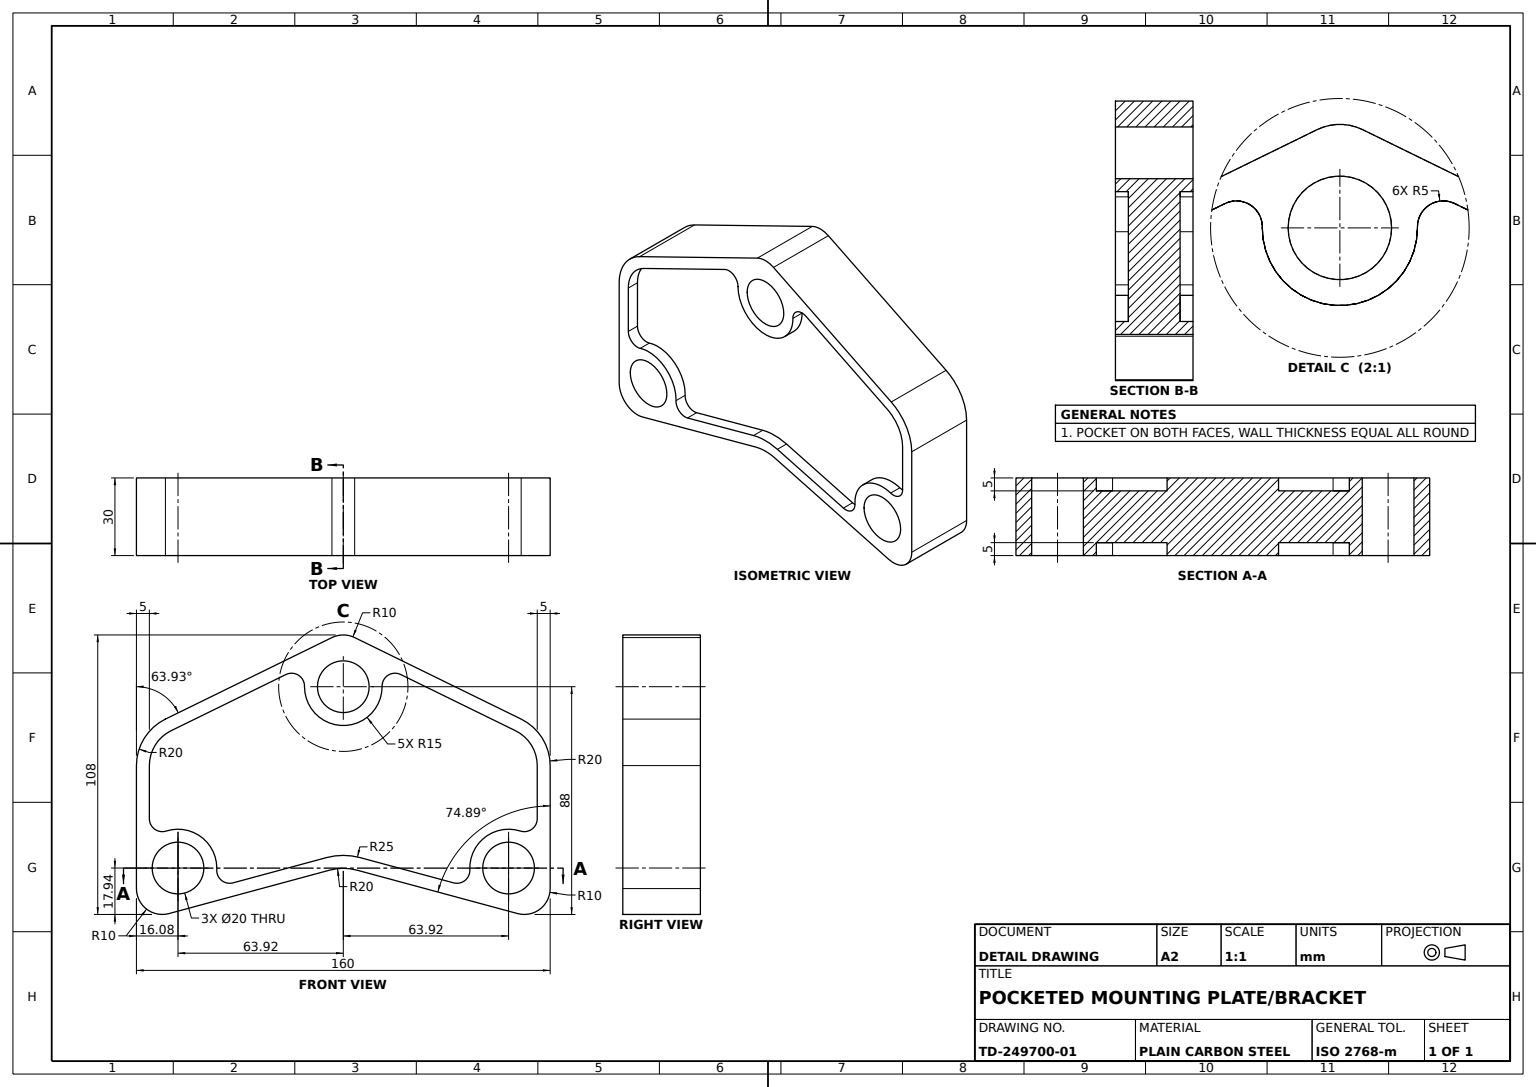
SolidWorks part; units mm, degrees
material "Plain Carbon Steel"
ref_plane "Front Plane" through (0, 0, 0) normal (0, 0, 1) x (1, 0, 0)
ref_plane "Top Plane" through (0, 0, 0) normal (0, 1, 0) x (1, 0, 0)
ref_plane "Right Plane" through (0, 0, 0) normal (1, 0, 0) x (0, 0, -1)
sketch "Bracket Outline Sketch" plane through (0, 0, 0) normal (0, 0, 1) x (1, 0, 0)
  line L0 (-36.0421, 0) -> (45.4547, 0) construction
  line L1 (0, 0) -> (0, -44) construction
  line L2 (-80, -88) -> (-80, -40.4814)
  line L3 (-68.788, -22.5156) -> (-4.394, 8.9829)
  line L4 (36.0421, 0) -> (-45.4547, 0) construction
  line L5 (68.788, -22.5156) -> (4.394, 8.9829)
  line L6 (80, -88) -> (80, -40.4814)
  line L7 (-104, -44) -> (91.1043, -44) construction
  line L8 (-67.3929, -97.6542) -> (-5.2143, -80.8627)
  line L9 (5.2143, -80.8627) -> (67.3929, -97.6542)
  arc A0 (4.394, 8.9829) -> (-4.394, 8.9829) centre (0, 0) ccw
  arc A1 (-80, -88) -> (-67.3929, -97.6542) centre (-70, -88) ccw
  arc A2 (67.3929, -97.6542) -> (80, -88) centre (70, -88) ccw
  arc A3 (-80, -40.4814) -> (-68.788, -22.5156) centre (-60, -40.4814) cw
  arc A4 (80, -40.4814) -> (68.788, -22.5156) centre (60, -40.4814) ccw
  arc A5 (-5.2143, -80.8627) -> (5.2143, -80.8627) centre (0, -100.171) cw
  point P16 (-80, -28)
  point P24 (80, -28)
  dimension "D1" = 20
  dimension "D2" = 20
  dimension "D3" = 100.171
  dimension "D8" = 20
  dimension "D10" = 20
  dimension "D4" = 88
  dimension "D5" = 140
  dimension "D6" = 70
  dimension "D7" = 60
  dimension "D9" = 44
extrude "Bracket Plate" add sketch "Bracket Outline Sketch" along normal mid plane 30
sketch "Face Pocket Sketch" plane through (0, 0, 15) normal (0, 0, 1) x (1, 0, 0)
  line L0 (80, -88) -> (80, -40.4814) construction
  line L1 (5.2143, -80.8627) -> (67.3929, -97.6542) construction
  line L2 (-67.3929, -97.6542) -> (-5.2143, -80.8627) construction
  line L3 (-80, -40.4814) -> (-80, -88) construction
  line L4 (68.788, -22.5156) -> (4.394, 8.9829) construction
  line L5 (-4.394, 8.9829) -> (-68.788, -22.5156) construction
  line L6 (80, -88) -> (80, -40.4814)
  line L7 (5.2143, -80.8627) -> (67.3929, -97.6542)
  line L8 (-67.3929, -97.6542) -> (-5.2143, -80.8627)
  line L9 (-80, -40.4814) -> (-80, -88)
  line L10 (68.788, -22.5156) -> (4.394, 8.9829)
  line L11 (-4.394, 8.9829) -> (-68.788, -22.5156)
  line L12 (75, -61.007) -> (75, -40.4814)
  line L13 (66.591, -27.0071) -> (22.1958, -5.291)
  line L14 (-22.1958, -5.291) -> (-66.591, -27.0071)
  line L15 (-75, -40.4814) -> (-75, -61.007)
  line L16 (-42.637, -85.7897) -> (-6.5178, -76.0356)
  line L17 (6.5178, -76.0356) -> (42.637, -85.7897)
  line L18 (0, 10) -> (0, -10) construction
  line L19 (-2.197, 4.4915) -> (-66.591, -27.0071) construction
  line L20 (66.591, -27.0071) -> (2.197, 4.4915) construction
  line L21 (-76.0798, -95.9395) -> (-63.9202, -80.0605) construction
  line L22 (-68.6964, -92.8271) -> (-6.5178, -76.0356) construction
  line L23 (-75, -40.4814) -> (-75, -88) construction
  line L24 (0, -100.171) -> (0, -54.8993) construction
  line L25 (6.5178, -76.0356) -> (68.6964, -92.8271) construction
  line L26 (75, -88) -> (75, -40.4814) construction
  arc A0 (80, -40.4814) -> (68.788, -22.5156) centre (60, -40.4814) ccw construction
  arc A1 (67.3929, -97.6542) -> (80, -88) centre (70, -88) ccw construction
  arc A2 (5.2143, -80.8627) -> (-5.2143, -80.8627) centre (0, -100.171) ccw construction
  arc A3 (-80, -88) -> (-67.3929, -97.6542) centre (-70, -88) ccw construction
  arc A4 (-68.788, -22.5156) -> (-80, -40.4814) centre (-60, -40.4814) ccw construction
  arc A5 (4.394, 8.9829) -> (-4.394, 8.9829) centre (0, 0) ccw construction
  arc A6 (80, -40.4814) -> (68.788, -22.5156) centre (60, -40.4814) ccw
  arc A7 (67.3929, -97.6542) -> (80, -88) centre (70, -88) ccw
  arc A8 (5.2143, -80.8627) -> (-5.2143, -80.8627) centre (0, -100.171) ccw
  arc A9 (-80, -88) -> (-67.3929, -97.6542) centre (-70, -88) ccw
  arc A10 (-68.788, -22.5156) -> (-80, -40.4814) centre (-60, -40.4814) ccw
  arc A11 (4.394, 8.9829) -> (-4.394, 8.9829) centre (0, 0) ccw
  arc A12 (75, -40.4814) -> (66.591, -27.0071) centre (60, -40.4814) ccw
  arc A14 (-66.591, -27.0071) -> (-75, -40.4814) centre (-60, -40.4814) ccw
  arc A16 (6.5178, -76.0356) -> (-6.5178, -76.0356) centre (0, -100.171) ccw
  circle A18 centre (0, -10) radius 10
  arc A19 (-14.9991, -9.8369) -> (14.9991, -9.8369) centre (0, -10) ccw
  arc A20 (-14.9991, -9.8369) -> (-22.1958, -5.291) centre (-19.9988, -9.7825) ccw
  arc A21 (14.9991, -9.8369) -> (22.1958, -5.291) centre (19.9988, -9.7825) cw
  arc A22 (2.197, 4.4915) -> (-2.197, 4.4915) centre (0, 0) ccw construction
  arc A24 (-48.9354, -80.7371) -> (-68.48, -65.7704) centre (-63.9202, -80.0605) ccw
  circle A25 centre (-63.9202, -80.0605) radius 10
  arc A26 (-75, -61.007) -> (-68.48, -65.7704) centre (-70, -61.007) ccw
  arc A27 (-48.9354, -80.7371) -> (-42.637, -85.7897) centre (-43.9405, -80.9626) ccw
  arc A28 (-75, -88) -> (-68.6964, -92.8271) centre (-70, -88) ccw construction
  arc A29 (48.9354, -80.7371) -> (42.637, -85.7897) centre (43.9405, -80.9626) cw
  arc A30 (48.9354, -80.7371) -> (68.48, -65.7704) centre (63.9202, -80.0605) cw
  arc A31 (75, -61.007) -> (68.48, -65.7704) centre (70, -61.007) cw
  circle A32 centre (63.9202, -80.0605) radius 10
  arc A33 (68.6964, -92.8271) -> (75, -88) centre (70, -88) ccw construction
  dimension "D3" = 30
  dimension "D4" = 20
  dimension "D5" = 5
  dimension "D6" = 20
  dimension "D7" = 30
  dimension "D8" = 20
  dimension "D9" = 5
  dimension "D10" = 5
  dimension "D2" = 20
  dimension "D1" = 5
extrude "Front Face Pocket" cut sketch "Face Pocket Sketch" against normal blind 5 contours L12 A12 L13 A21 A19 A20 L14 A14 L15 A26 A24 A27 L16 A16 L17 A29 A30 A31
ref_plane "Pocket Mirror Plane" through (0, 0, 0) normal (0, 0, 1) x (1, 0, 0)
mirror "Back Face Pocket Mirror" about plane through (0, 0, 0) normal (0, 0, 1) of "Front Face Pocket"
sketch "Mounting Holes Sketch" plane through (0, 0, 10) normal (0, 0, 1) x (1, 0, 0)
  arc A0 (68.48, -65.7704) -> (48.9354, -80.7371) centre (63.9202, -80.0605) ccw construction
  arc A1 (-14.9991, -9.8369) -> (14.9991, -9.8369) centre (0, -10) ccw construction
  arc A2 (-48.9354, -80.7371) -> (-68.48, -65.7704) centre (-63.9202, -80.0605) ccw construction
  arc A3 (68.48, -65.7704) -> (48.9354, -80.7371) centre (63.9202, -80.0605) ccw
  arc A4 (-14.9991, -9.8369) -> (14.9991, -9.8369) centre (0, -10) ccw
  arc A5 (-48.9354, -80.7371) -> (-68.48, -65.7704) centre (-63.9202, -80.0605) ccw
  circle A6 centre (-63.9202, -80.0605) radius 10
  circle A7 centre (0, -10) radius 10
  circle A8 centre (63.9202, -80.0605) radius 10
  dimension "D1" = 20
  dimension "D2" = 20
  dimension "D3" = 20
extrude "Mounting Holes x3" cut sketch "Mounting Holes Sketch" against normal through all both and the other way through all contours A6 | A7 | A8
